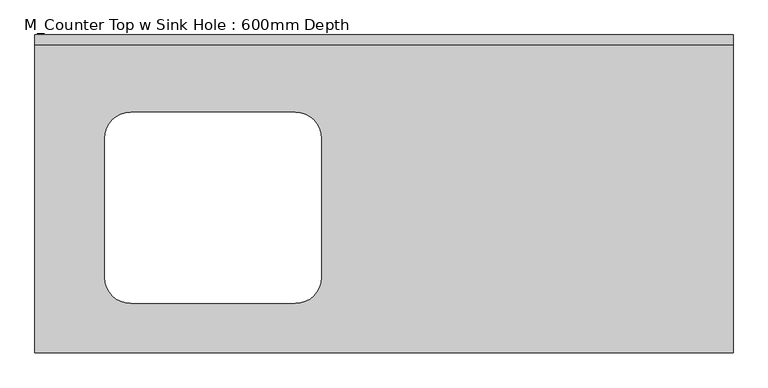
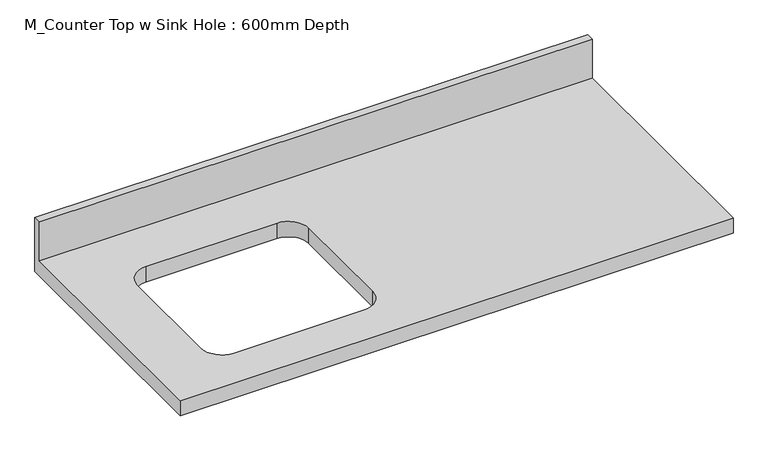
"""IFC4 building model written with IfcOpenShell, lengths in millimetres: furniture geometry, M_Counter Top w Sink Hole : 600mm Depth."""

from ifc_helpers import new_model, si_unit, frame, origin, place, context, project, spatial, polyline, circle_curve, source, transform, mapped, element, save
from ifc_brep_helpers import plane_surface, revolved_surface, advanced_brep


def m_counter_top_w_sink_hole_600mm_depth_edbb3572(model_context):
    return source(origin(), model_context, "Body", "AdvancedBrep", [
        advanced_brep(
        [(-1200.4622951, -625.0, 900.0), (171.5377049, -625.0, 900.0), (171.5377049, -19.05, 900.0), (-1200.4622951, -19.05, 900.0), (-1012.3622951, -152.3, 900.0), (-688.5622951, -152.3, 900.0), (-637.7622951, -203.1, 900.0), (-637.7622951, -476.9, 900.0), (-688.5622951, -527.7, 900.0), (-1012.3622951, -527.7, 900.0), (-1063.1622951, -476.9, 900.0), (-1063.1622951, -203.1, 900.0), (171.5377049, 0.0, 860.0), (171.5377049, -625.0, 860.0), (-1200.4622951, -625.0, 860.0), (-1200.4622951, 0.0, 860.0), (-688.5622951, -152.3, 860.0), (-1012.3622951, -152.3, 860.0), (-1063.1622951, -203.1, 860.0), (-1063.1622951, -476.9, 860.0), (-1012.3622951, -527.7, 860.0), (-688.5622951, -527.7, 860.0), (-637.7622951, -476.9, 860.0), (-637.7622951, -203.1, 860.0), (-1200.4622951, 0.0, 1001.6), (171.5377049, 0.0, 1001.6), (-1200.4622951, -19.05, 1001.6), (171.5377049, -19.05, 1001.6)],
        [
            (0, 1),
            (1, 2),
            (2, 3),
            (3, 0),
            (4, 5),
            (5, 6, circle_curve(frame((-688.5622951, -203.1, 900.0), z_axis=(0.0, 0.0, -1.0), x_axis=(1.0, 0.0, 0.0)), 50.8)),
            (6, 7),
            (7, 8, circle_curve(frame((-688.5622951, -476.9, 900.0), z_axis=(0.0, 0.0, -1.0), x_axis=(1.0, 0.0, 0.0)), 50.8)),
            (8, 9),
            (9, 10, circle_curve(frame((-1012.3622951, -476.9, 900.0), z_axis=(0.0, 0.0, -1.0), x_axis=(1.0, 0.0, 0.0)), 50.8)),
            (10, 11),
            (11, 4, circle_curve(frame((-1012.3622951, -203.1, 900.0), z_axis=(0.0, 0.0, -1.0), x_axis=(1.0, 0.0, 0.0)), 50.8)),
            (12, 13),
            (13, 14),
            (14, 15),
            (15, 12),
            (16, 17),
            (17, 18, circle_curve(frame((-1012.3622951, -203.1, 860.0), z_axis=(0.0, 0.0, 1.0), x_axis=(1.0, 0.0, 0.0)), 50.8)),
            (18, 19),
            (19, 20, circle_curve(frame((-1012.3622951, -476.9, 860.0), z_axis=(0.0, 0.0, 1.0), x_axis=(1.0, 0.0, 0.0)), 50.8)),
            (20, 21),
            (21, 22, circle_curve(frame((-688.5622951, -476.9, 860.0), z_axis=(0.0, 0.0, 1.0), x_axis=(1.0, 0.0, 0.0)), 50.8)),
            (22, 23),
            (23, 16, circle_curve(frame((-688.5622951, -203.1, 860.0), z_axis=(0.0, 0.0, 1.0), x_axis=(1.0, 0.0, 0.0)), 50.8)),
            (15, 24),
            (24, 25),
            (25, 12),
            (14, 0),
            (3, 26),
            (26, 24),
            (13, 1),
            (25, 27),
            (27, 2),
            (26, 27),
            (4, 17),
            (16, 5),
            (11, 18),
            (10, 19),
            (9, 20),
            (8, 21),
            (7, 22),
            (6, 23),
        ],
        [
            plane_surface(frame((-1200.4622951, 0.0, 900.0), z_axis=(0.0, 0.0, 1.0), x_axis=(-1.0, 0.0, 0.0))),
            plane_surface(frame((-1200.4622951, 0.0, 860.0), z_axis=(0.0, 0.0, -1.0), x_axis=(1.0, 0.0, 0.0))),
            plane_surface(frame((171.5377049, 0.0, 900.0), z_axis=(0.0, 1.0, 0.0), x_axis=(0.0, 0.0, -1.0))),
            plane_surface(frame((-1200.4622951, 0.0, 900.0), z_axis=(-1.0, 0.0, 0.0), x_axis=(0.0, 0.0, -1.0))),
            plane_surface(frame((-1200.4622951, -625.0, 900.0), z_axis=(0.0, -1.0, 0.0), x_axis=(0.0, 0.0, -1.0))),
            plane_surface(frame((171.5377049, -625.0, 900.0), z_axis=(1.0, 0.0, 0.0), x_axis=(0.0, 0.0, -1.0))),
            plane_surface(frame((-1200.4622951, 0.0, 1001.6), z_axis=(0.0, 0.0, 1.0), x_axis=(0.0, -1.0, 0.0))),
            plane_surface(frame((-1200.4622951, -19.05, 1001.6), z_axis=(0.0, -1.0, 0.0), x_axis=(0.0, 0.0, -1.0))),
            plane_surface(frame((-688.5622951, -152.3, 900.0), z_axis=(0.0, -1.0, 0.0), x_axis=(0.0, 0.0, -1.0))),
            revolved_surface(polyline([(-961.5622951, -203.1, 900.0), (-961.5622951, -203.1, 860.0)]), (-1012.3622951, -203.1, 860.0), (0.0, 0.0, 1.0)),
            plane_surface(frame((-1063.1622951, -203.1, 900.0), z_axis=(1.0, 0.0, 0.0), x_axis=(0.0, 0.0, -1.0))),
            revolved_surface(polyline([(-961.5622951, -476.9, 900.0), (-961.5622951, -476.9, 860.0)]), (-1012.3622951, -476.9, 860.0), (0.0, 0.0, 1.0)),
            plane_surface(frame((-1012.3622951, -527.7, 900.0), z_axis=(0.0, 1.0, 0.0), x_axis=(0.0, 0.0, -1.0))),
            revolved_surface(polyline([(-637.7622951000001, -476.9, 900.0), (-637.7622951000001, -476.9, 860.0)]), (-688.5622951, -476.9, 860.0), (0.0, 0.0, 1.0)),
            plane_surface(frame((-637.7622951, -476.9, 900.0), z_axis=(-1.0, 0.0, 0.0), x_axis=(0.0, 0.0, -1.0))),
            revolved_surface(polyline([(-637.7622951000001, -203.1, 900.0), (-637.7622951000001, -203.1, 860.0)]), (-688.5622951, -203.1, 860.0), (0.0, 0.0, 1.0)),
        ],
        [
            (0, [[1, 2, 3, 4], [5, 6, 7, 8, 9, 10, 11, 12]]),
            (1, [[13, 14, 15, 16], [17, 18, 19, 20, 21, 22, 23, 24]]),
            (2, [[-16, 25, 26, 27]]),
            (3, [[-15, 28, -4, 29, 30, -25]]),
            (4, [[-1, -28, -14, 31]]),
            (5, [[-13, -27, 32, 33, -2, -31]]),
            (6, [[-30, 34, -32, -26]]),
            (7, [[-34, -29, -3, -33]]),
            (8, [[35, -17, 36, -5]]),
            (9, [[-35, -12, 37, -18]]),
            (10, [[-37, -11, 38, -19]]),
            (11, [[-38, -10, 39, -20]]),
            (12, [[-39, -9, 40, -21]]),
            (13, [[-40, -8, 41, -22]]),
            (14, [[-41, -7, 42, -23]]),
            (15, [[-36, -24, -42, -6]]),
        ],
    ),
    ])


if __name__ == "__main__":
    model = new_model("IFC4")
    model_context = context("Model", 3, world=origin())
    ifc_project = project(units=[si_unit("LENGTHUNIT", "METRE", prefix="MILLI")], contexts=[model_context])
    site = spatial("IfcSite", under=ifc_project)
    building = spatial("IfcBuilding", under=site)
    placement = place(None, origin())
    m_counter_top_w_sink_hole_600mm_depth_shape = m_counter_top_w_sink_hole_600mm_depth_edbb3572(model_context)
    element("IfcFurniture", 1, ObjectType="M_Counter Top w Sink Hole : 600mm Depth", at=placement, inside=building, context=model_context, shape_type="MappedRepresentation", body=[
        mapped(m_counter_top_w_sink_hole_600mm_depth_shape, transform((0.0, 0.0, 0.0), x_axis=(1.0, 0.0, 0.0), y_axis=(0.0, 1.0, 0.0), z_axis=(0.0, 0.0, 1.0))),
    ])
    save(model, "model.ifc")

# Revit data of these elements
# Type "M_Counter Top w Sink Hole : 600mm Depth"
#   Counter Thickness = 40 mm
#   Depth = 625 mm
#   Height = 900 mm
#   Length [instance default] = 2500 mm
#   Sink Location [instance default] = 1200 mm
#   Sink Location To Wall [instance default] = 100 mm
#   Sink Opening Depth [instance default] = 378 mm
#   Sink Opening Width [instance default] = 587 mm
#   Counter Top Material = none
#   Default Elevation = 0
# Element 1 (IfcFurniture, "M_Counter Top w Sink Hole : 600mm Depth")
#   Length = 1372 mm
#   Sink Location = 350 mm
#   Sink Location To Wall = 165 mm
#   Sink Opening Depth = 350 mm
#   Sink Opening Width = 400 mm
#   Materials on its faces: "Counter Top"
# Materials
#   "Counter Top": class "Wood", colour RGB 226 177 128, transparency 0
